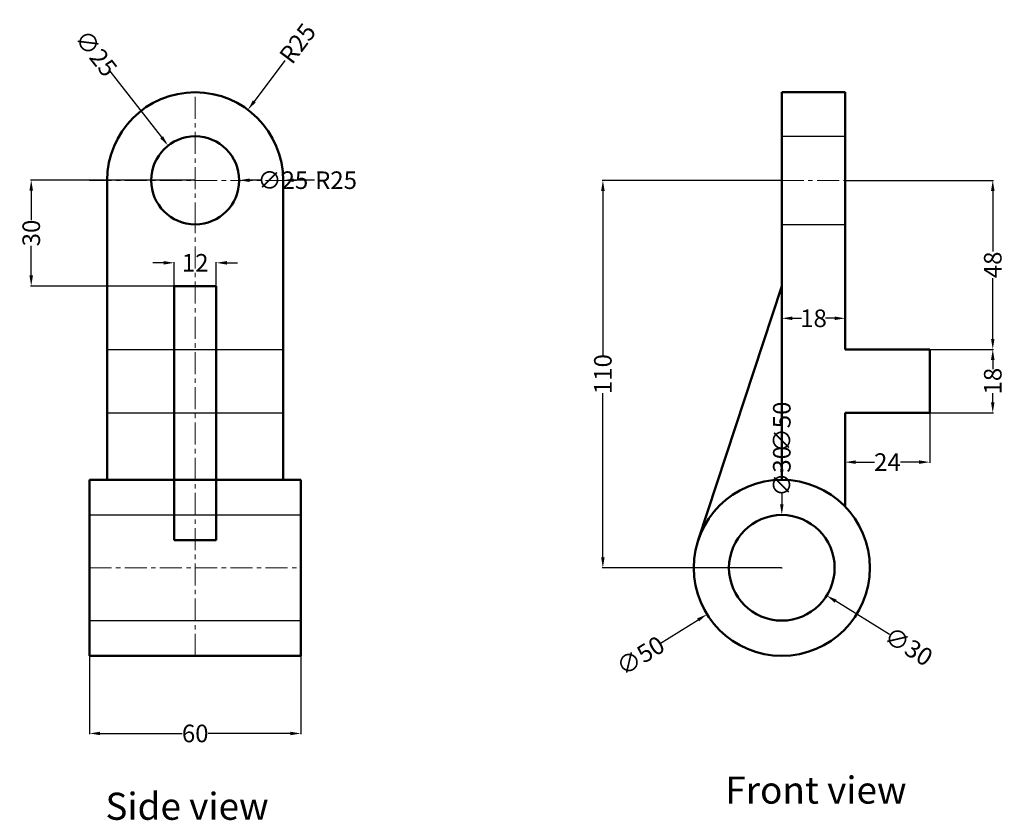
# Model space of a CAD drawing. Units: inches. Extents: x 36 to 316, y 40 to 267.
import ezdxf

# ---------------------------------------------------------------- set-up
doc = ezdxf.new("R2010")
doc.units = ezdxf.units.IN
doc.header["$MEASUREMENT"] = 0
doc.linetypes.add('CENTER', pattern=[2, 1.25, -0.25, 0.25, -0.25])
doc.linetypes.add('HIDDEN', pattern=[9.525, 6.35, -3.175])
for name, color, linetype, lineweight in [('M-CNTR', 4, 'CENTER', 18), ('M-DIMS', 2, 'Continuous', 25), ('M-HIDN', 3, 'HIDDEN', 25), ('M-OUTL', 7, 'Continuous', 50), ('M-TEXT', 7, 'Continuous', 25)]:
    doc.layers.add(name, color=color, linetype=linetype, lineweight=lineweight)
doc.styles.get("Standard").update_dxf_attribs({"font": 'arial.ttf'})
doc.dimstyles.get("Standard").update_dxf_attribs({"dimtxt": 5, "dimasz": 3, "dimexe": 0.18, "dimexo": 0.0625, "dimgap": 0.09, "dimtad": 0, "dimdec": 0, "dimzin": 0, "dimdsep": 46, "dimtxsty": 'Standard', "dimcen": 0.09, "dimadec": 0, "dimazin": 0, "dimtfac": 1, "dimtdec": 0, "dimtofl": 0, "dimtmove": 0, "dimatfit": 3, "dimfxl": 1, "dimtolj": 1, "dimtzin": 0, "dimarcsym": 0})

# ---------------------------------------------------------------- blocks, each defined once
blk = doc.blocks.new('*D1')
at = {"layer": 'Defpoints', "color": 0, "transparency": 16777216}
for p in [(252.72, 221.19), (201.9, 111.19), (252.72, 111.19)]:
    blk.add_point(p, dxfattribs=at)
at = {"layer": 'M-DIMS', "color": 0, "lineweight": -2, "transparency": 16777216}
for p, q in [((252.66, 221.19), (201.72, 221.19)), ((201.9, 218.19), (201.9, 171.56)), ((201.9, 114.19), (201.9, 160.82)), ((252.66, 111.19), (201.72, 111.19))]:
    blk.add_line(p, q, dxfattribs=at)
at = {"layer": 'M-DIMS', "color": 0, "transparency": 16777216}
for points in [[(201.4, 218.19), (202.4, 218.19), (201.9, 221.19)], [(201.4, 114.19), (202.4, 114.19), (201.9, 111.19)]]:
    blk.add_solid(points, dxfattribs=at)
at = {"layer": 'M-DIMS', "color": 0, "transparency": 16777216, "insert": (201.9, 166.19), "char_height": 5, "attachment_point": 5, "rotation": 90}
blk.add_mtext('\\A1;110', dxfattribs=at)
blk = doc.blocks.new('*D2')
at = {"layer": 'Defpoints', "color": 0, "transparency": 16777216}
for p in [(273.96, 124.39), (231.49, 98)]:
    blk.add_point(p, dxfattribs=at)
at = {"layer": 'M-DIMS', "color": 0, "lineweight": -2, "transparency": 16777216}
for p, q in [((252.63, 111.19), (252.81, 111.19)), ((252.72, 111.1), (252.72, 111.28)), ((217.99, 89.61), (228.94, 96.41))]:
    blk.add_line(p, q, dxfattribs=at)
at = {"layer": 'M-DIMS', "color": 0, "transparency": 16777216}
blk.add_solid([(228.68, 96.84), (229.2, 95.99), (231.49, 98)], dxfattribs=at)
at = {"layer": 'M-DIMS', "color": 0, "transparency": 16777216, "insert": (212.57, 86.24), "char_height": 5, "attachment_point": 5, "rotation": 31.8568}
blk.add_mtext('\\A1;∅50', dxfattribs=at)
blk = doc.blocks.new('*D3')
at = {"layer": 'Defpoints', "color": 0, "transparency": 16777216}
for p in [(239.97, 119.09), (265.48, 103.3)]:
    blk.add_point(p, dxfattribs=at)
at = {"layer": 'M-DIMS', "color": 0, "lineweight": -2, "transparency": 16777216}
for p, q in [((252.63, 111.19), (252.81, 111.19)), ((252.72, 111.1), (252.72, 111.28)), ((283.31, 92.25), (268.03, 101.72))]:
    blk.add_line(p, q, dxfattribs=at)
at = {"layer": 'M-DIMS', "color": 0, "transparency": 16777216}
blk.add_solid([(268.29, 102.14), (267.76, 101.29), (265.48, 103.3)], dxfattribs=at)
at = {"layer": 'M-DIMS', "color": 0, "transparency": 16777216, "insert": (288.74, 88.89), "char_height": 5, "attachment_point": 5, "rotation": 328.2295}
blk.add_mtext('\\A1;∅30', dxfattribs=at)
blk = doc.blocks.new('*D4')
at = {"layer": 'Defpoints', "color": 0, "transparency": 16777216}
for p in [(294.72, 173.19), (312.64, 173.19), (294.72, 155.19)]:
    blk.add_point(p, dxfattribs=at)
at = {"layer": 'M-DIMS', "color": 0, "lineweight": -2, "transparency": 16777216}
for p, q in [((294.79, 173.19), (312.82, 173.19)), ((312.64, 170.19), (312.64, 167.63)), ((312.64, 158.19), (312.64, 160.75)), ((294.79, 155.19), (312.82, 155.19))]:
    blk.add_line(p, q, dxfattribs=at)
at = {"layer": 'M-DIMS', "color": 0, "transparency": 16777216}
for points in [[(312.14, 170.19), (313.14, 170.19), (312.64, 173.19)], [(312.14, 158.19), (313.14, 158.19), (312.64, 155.19)]]:
    blk.add_solid(points, dxfattribs=at)
at = {"layer": 'M-DIMS', "color": 0, "transparency": 16777216, "insert": (312.64, 164.19), "char_height": 5, "attachment_point": 5, "rotation": 90}
blk.add_mtext('\\A1;18', dxfattribs=at)
blk = doc.blocks.new('*D5')
at = {"layer": 'Defpoints', "color": 0, "transparency": 16777216}
for p in [(270.72, 155.19), (294.72, 155.19), (294.72, 141.2)]:
    blk.add_point(p, dxfattribs=at)
at = {"layer": 'M-DIMS', "color": 0, "lineweight": -2, "transparency": 16777216}
for p, q in [((270.72, 155.13), (270.72, 141.02)), ((294.72, 155.13), (294.72, 141.02)), ((273.72, 141.2), (279.02, 141.2)), ((291.72, 141.2), (286.43, 141.2))]:
    blk.add_line(p, q, dxfattribs=at)
at = {"layer": 'M-DIMS', "color": 0, "transparency": 16777216}
for points in [[(273.72, 141.7), (273.72, 140.7), (270.72, 141.2)], [(291.72, 141.7), (291.72, 140.7), (294.72, 141.2)]]:
    blk.add_solid(points, dxfattribs=at)
at = {"layer": 'M-DIMS', "color": 0, "transparency": 16777216, "insert": (282.72, 141.2), "char_height": 5, "attachment_point": 5}
blk.add_mtext('\\A1;24', dxfattribs=at)
blk = doc.blocks.new('*D6')
at = {"layer": 'Defpoints', "color": 0, "transparency": 16777216}
for p in [(270.72, 221.19), (270.72, 173.19), (312.64, 173.19)]:
    blk.add_point(p, dxfattribs=at)
at = {"layer": 'M-DIMS', "color": 0, "lineweight": -2, "transparency": 16777216}
for p, q in [((270.79, 221.19), (312.82, 221.19)), ((312.64, 218.19), (312.64, 200.97)), ((312.64, 176.19), (312.64, 193.42)), ((270.79, 173.19), (312.82, 173.19))]:
    blk.add_line(p, q, dxfattribs=at)
at = {"layer": 'M-DIMS', "color": 0, "transparency": 16777216}
for points in [[(312.14, 218.19), (313.14, 218.19), (312.64, 221.19)], [(312.14, 176.19), (313.14, 176.19), (312.64, 173.19)]]:
    blk.add_solid(points, dxfattribs=at)
at = {"layer": 'M-DIMS', "color": 0, "transparency": 16777216, "insert": (312.64, 197.19), "char_height": 5, "attachment_point": 5, "rotation": 90}
blk.add_mtext('\\A1;48', dxfattribs=at)
blk = doc.blocks.new('*D7')
at = {"layer": 'Defpoints', "color": 0, "transparency": 16777216}
for p in [(252.72, 182.03), (252.72, 173.19), (270.72, 173.19)]:
    blk.add_point(p, dxfattribs=at)
at = {"layer": 'M-DIMS', "color": 0, "lineweight": -2, "transparency": 16777216}
for p, q in [((252.72, 173.26), (252.72, 182.21)), ((255.72, 182.03), (258.28, 182.03)), ((267.72, 182.03), (265.16, 182.03)), ((270.72, 173.26), (270.72, 182.21))]:
    blk.add_line(p, q, dxfattribs=at)
at = {"layer": 'M-DIMS', "color": 0, "transparency": 16777216}
for points in [[(255.72, 182.53), (255.72, 181.53), (252.72, 182.03)], [(267.72, 182.53), (267.72, 181.53), (270.72, 182.03)]]:
    blk.add_solid(points, dxfattribs=at)
at = {"layer": 'M-DIMS', "color": 0, "transparency": 16777216, "insert": (261.72, 182.03), "char_height": 5, "attachment_point": 5}
blk.add_mtext('\\A1;18', dxfattribs=at)
blk = doc.blocks.new('*D8')
at = {"layer": 'Defpoints', "color": 0, "transparency": 16777216}
for p in [(101.09, 241.21), (86.11, 221.19)]:
    blk.add_point(p, dxfattribs=at)
at = {"layer": 'M-DIMS', "color": 0, "lineweight": -2, "transparency": 16777216}
for p, q in [((111.56, 255.2), (102.89, 243.61)), ((86.02, 221.19), (86.2, 221.19)), ((86.11, 221.1), (86.11, 221.28))]:
    blk.add_line(p, q, dxfattribs=at)
at = {"layer": 'M-DIMS', "color": 0, "transparency": 16777216}
blk.add_solid([(102.49, 243.91), (103.29, 243.31), (101.09, 241.21)], dxfattribs=at)
at = {"layer": 'M-DIMS', "color": 0, "transparency": 16777216, "insert": (115.2, 260.07), "char_height": 5, "attachment_point": 5, "rotation": 53.1928}
blk.add_mtext('\\A1;R25', dxfattribs=at)
blk = doc.blocks.new('*D9')
at = {"layer": 'Defpoints', "color": 0, "transparency": 16777216}
for p in [(78.42, 231.05), (93.81, 211.34)]:
    blk.add_point(p, dxfattribs=at)
at = {"layer": 'M-DIMS', "color": 0, "lineweight": -2, "transparency": 16777216}
for p, q in [((61.89, 252.22), (76.58, 233.41)), ((86.02, 221.19), (86.2, 221.19)), ((86.11, 221.1), (86.11, 221.28))]:
    blk.add_line(p, q, dxfattribs=at)
at = {"layer": 'M-DIMS', "color": 0, "transparency": 16777216}
blk.add_solid([(76.97, 233.72), (76.18, 233.1), (78.42, 231.05)], dxfattribs=at)
at = {"layer": 'M-DIMS', "color": 0, "transparency": 16777216, "insert": (57.95, 257.27), "char_height": 5, "attachment_point": 5, "rotation": 307.9788}
blk.add_mtext('\\A1;∅25', dxfattribs=at)
blk = doc.blocks.new('*D10')
at = {"layer": 'Defpoints', "color": 0, "transparency": 16777216}
for p in [(86.11, 221.28), (39.54, 191.19), (86.11, 191.19)]:
    blk.add_point(p, dxfattribs=at)
at = {"layer": 'M-DIMS', "color": 0, "lineweight": -2, "transparency": 16777216}
for p, q in [((86.05, 221.28), (39.36, 221.28)), ((39.54, 218.28), (39.54, 209.9)), ((39.54, 194.19), (39.54, 202.58)), ((86.05, 191.19), (39.36, 191.19))]:
    blk.add_line(p, q, dxfattribs=at)
at = {"layer": 'M-DIMS', "color": 0, "transparency": 16777216}
for points in [[(39.04, 218.28), (40.04, 218.28), (39.54, 221.28)], [(39.04, 194.19), (40.04, 194.19), (39.54, 191.19)]]:
    blk.add_solid(points, dxfattribs=at)
at = {"layer": 'M-DIMS', "color": 0, "transparency": 16777216, "insert": (39.54, 206.24), "char_height": 5, "attachment_point": 5, "rotation": 90}
blk.add_mtext('\\A1;30', dxfattribs=at)
blk = doc.blocks.new('*D11')
at = {"layer": 'Defpoints', "color": 0, "transparency": 16777216}
for p in [(92.11, 197.78), (80.11, 191.19), (92.11, 191.19)]:
    blk.add_point(p, dxfattribs=at)
at = {"layer": 'M-DIMS', "color": 0, "lineweight": -2, "transparency": 16777216}
for p, q in [((77.11, 197.78), (74.11, 197.78)), ((80.11, 191.26), (80.11, 197.96)), ((92.11, 191.26), (92.11, 197.96)), ((95.11, 197.78), (98.11, 197.78))]:
    blk.add_line(p, q, dxfattribs=at)
at = {"layer": 'M-DIMS', "color": 0, "transparency": 16777216}
for points in [[(77.11, 198.28), (77.11, 197.28), (80.11, 197.78)], [(95.11, 198.28), (95.11, 197.28), (92.11, 197.78)]]:
    blk.add_solid(points, dxfattribs=at)
at = {"layer": 'M-DIMS', "color": 0, "transparency": 16777216, "insert": (86.11, 197.78), "char_height": 5, "attachment_point": 5}
blk.add_mtext('\\A1;12', dxfattribs=at)
blk = doc.blocks.new('*D12')
at = {"layer": 'Defpoints', "color": 0, "transparency": 16777216}
for p in [(56.11, 86.19), (116.11, 86.19), (116.11, 64.17)]:
    blk.add_point(p, dxfattribs=at)
at = {"layer": 'M-DIMS', "color": 0, "lineweight": -2, "transparency": 16777216}
for p, q in [((56.11, 86.13), (56.11, 63.99)), ((116.11, 86.13), (116.11, 63.99)), ((59.11, 64.17), (82.44, 64.17)), ((113.11, 64.17), (89.79, 64.17))]:
    blk.add_line(p, q, dxfattribs=at)
at = {"layer": 'M-DIMS', "color": 0, "transparency": 16777216}
for points in [[(59.11, 64.67), (59.11, 63.67), (56.11, 64.17)], [(113.11, 64.67), (113.11, 63.67), (116.11, 64.17)]]:
    blk.add_solid(points, dxfattribs=at)
at = {"layer": 'M-DIMS', "color": 0, "transparency": 16777216, "insert": (86.11, 64.17), "char_height": 5, "attachment_point": 5}
blk.add_mtext('\\A1;60', dxfattribs=at)
blk = doc.blocks.new('*D13')
at = {"layer": 'Defpoints', "color": 0, "transparency": 16777216}
for p in [(86.11, 221.19), (111.11, 221.22)]:
    blk.add_point(p, dxfattribs=at)
at = {"layer": 'M-DIMS', "color": 0, "lineweight": -2, "transparency": 16777216}
for p, q in [((86.02, 221.19), (86.2, 221.19)), ((86.11, 221.1), (86.11, 221.28)), ((120.03, 221.22), (114.11, 221.22))]:
    blk.add_line(p, q, dxfattribs=at)
at = {"layer": 'M-DIMS', "color": 0, "transparency": 16777216}
blk.add_solid([(114.11, 221.72), (114.12, 220.72), (111.11, 221.22)], dxfattribs=at)
at = {"layer": 'M-DIMS', "color": 0, "transparency": 16777216, "insert": (126.11, 221.23), "char_height": 5, "attachment_point": 5, "rotation": 0.0502}
blk.add_mtext('\\A1;R25', dxfattribs=at)
blk = doc.blocks.new('*D14')
at = {"layer": 'Defpoints', "color": 0, "transparency": 16777216}
for p in [(73.61, 221.17), (98.61, 221.21)]:
    blk.add_point(p, dxfattribs=at)
at = {"layer": 'M-DIMS', "color": 0, "lineweight": -2, "transparency": 16777216}
for p, q in [((86.02, 221.19), (86.2, 221.19)), ((86.11, 221.1), (86.11, 221.28)), ((104.61, 221.23), (101.61, 221.22))]:
    blk.add_line(p, q, dxfattribs=at)
at = {"layer": 'M-DIMS', "color": 0, "transparency": 16777216}
blk.add_solid([(101.61, 221.72), (101.62, 220.72), (98.61, 221.21)], dxfattribs=at)
at = {"layer": 'M-DIMS', "color": 0, "transparency": 16777216, "insert": (111.02, 221.24), "char_height": 5, "attachment_point": 5, "rotation": 0.1004}
blk.add_mtext('\\A1;∅25', dxfattribs=at)
blk = doc.blocks.new('*D15')
at = {"layer": 'Defpoints', "color": 0, "transparency": 16777216}
for p in [(252.72, 136.19), (252.72, 86.19)]:
    blk.add_point(p, dxfattribs=at)
at = {"layer": 'M-DIMS', "color": 0, "lineweight": -2, "transparency": 16777216}
for p, q in [((252.72, 144.81), (252.72, 139.19)), ((252.63, 111.19), (252.81, 111.19)), ((252.72, 111.1), (252.72, 111.28))]:
    blk.add_line(p, q, dxfattribs=at)
at = {"layer": 'M-DIMS', "color": 0, "transparency": 16777216}
blk.add_solid([(252.22, 139.19), (253.22, 139.19), (252.72, 136.19)], dxfattribs=at)
at = {"layer": 'M-DIMS', "color": 0, "transparency": 16777216, "insert": (252.72, 151.19), "char_height": 5, "attachment_point": 5, "rotation": 89.9996}
blk.add_mtext('\\A1;∅50', dxfattribs=at)
blk = doc.blocks.new('*D16')
at = {"layer": 'Defpoints', "color": 0, "transparency": 16777216}
for p in [(252.72, 126.19), (252.72, 96.19)]:
    blk.add_point(p, dxfattribs=at)
at = {"layer": 'M-DIMS', "color": 0, "lineweight": -2, "transparency": 16777216}
for p, q in [((252.72, 132.19), (252.72, 129.19)), ((252.63, 111.19), (252.81, 111.19)), ((252.72, 111.1), (252.72, 111.28))]:
    blk.add_line(p, q, dxfattribs=at)
at = {"layer": 'M-DIMS', "color": 0, "transparency": 16777216}
blk.add_solid([(252.22, 129.19), (253.22, 129.19), (252.72, 126.19)], dxfattribs=at)
at = {"layer": 'M-DIMS', "color": 0, "transparency": 16777216, "insert": (252.72, 138.58), "char_height": 5, "attachment_point": 5, "rotation": 89.9993}
blk.add_mtext('\\A1;∅30', dxfattribs=at)

msp = doc.modelspace()

# ---------------------------------------------------------------- linework, layer by layer
at = {"layer": 'M-CNTR', "ltscale": 5}
for p, q in [((86.11, 208.69), (86.11, 246.19)), ((56.11, 221.19), (116.11, 221.19)), ((252.72, 221.19), (270.72, 221.19)), ((86.11, 86.19), (86.11, 208.69)), ((56.11, 111.19), (116.11, 111.19))]:
    msp.add_line(p, q, dxfattribs=at)
at = {"layer": 'M-HIDN', "ltscale": 10}
for p, q in [((252.72, 233.69), (270.72, 233.69)), ((252.72, 208.69), (270.72, 208.69)), ((61.11, 173.19), (111.11, 173.19)), ((61.11, 155.19), (111.11, 155.19)), ((56.11, 126.19), (116.11, 126.19)), ((56.11, 96.19), (116.11, 96.19))]:
    msp.add_line(p, q, dxfattribs=at)
at = {"layer": 'M-OUTL'}
for p, q in [((252.72, 136.19), (252.72, 246.19)), ((252.72, 246.19), (270.72, 246.19)), ((270.72, 173.19), (270.72, 246.19)), ((61.11, 136.19), (61.11, 221.19)), ((111.11, 136.19), (111.11, 221.19)), ((92.11, 191.19), (80.11, 191.19)), ((80.11, 119.01), (80.11, 191.19)), ((92.11, 119.01), (92.11, 191.19)), ((252.72, 191.19), (228.97, 119.01)), ((270.72, 173.19), (294.72, 173.19)), ((294.72, 155.19), (294.72, 173.19)), ((270.72, 128.54), (270.72, 155.19)), ((270.72, 155.19), (294.72, 155.19)), ((56.11, 86.19), (56.11, 136.19)), ((56.11, 136.19), (116.11, 136.19)), ((116.11, 86.19), (116.11, 136.19)), ((92.11, 119.01), (80.11, 119.01)), ((56.11, 86.19), (116.11, 86.19))]:
    msp.add_line(p, q, dxfattribs=at)
for centre, radius in [((86.11, 221.19), 12.5), ((252.72, 111.19), 25), ((252.72, 111.19), 15)]:
    msp.add_circle(centre, radius, dxfattribs=at)
for start, end in [(90, 180), (0, 90)]:
    msp.add_arc((86.11, 221.19), 25, start, end, dxfattribs=at)

# ---------------------------------------------------------------- texts
at = {"layer": 'M-TEXT', "char_height": 7.685, "attachment_point": 1}
for s, insert in [('Front view', (236.69, 51.93)), ('Side view', (60.61, 47.34))]:
    msp.add_mtext_dynamic_manual_height_columns(s, width=75.585, gutter_width=0.769, heights=[0], dxfattribs=dict(at, insert=insert))

# ---------------------------------------------------------------- dimensions: what is measured, and where the dimension line sits
at = {"layer": 'M-DIMS'}
for mpoint, override, picture, middle in [((101.09, 241.21), {"dimclrd": 0, "dimclre": 0, "dimclrt": 0}, '*D8', (115.2, 260.07)), ((111.11, 221.21), {"dimdec": 0, "dimlfac": 1, "dimrnd": 0, "dimzin": 0, "dimdsep": 46, "dimlunit": 2}, '*D13', (126.11, 221.23))]:
    dim = msp.add_radius_dim(center=(86.11, 221.19), mpoint=mpoint, dimstyle='Standard', override=override, dxfattribs=at)
    dim.commit()
    dim.dimension.update_dxf_attribs({"geometry": picture, "text_midpoint": middle, "dimtype": 164})
for p1, p2, override, picture, middle in [((93.81, 211.34), (78.42, 231.05), {"dimclrd": 0, "dimclre": 0, "dimclrt": 0}, '*D9', (57.95, 257.27)), ((252.72, 86.19), (252.72, 136.19), {"dimdec": 0, "dimlfac": 1, "dimrnd": 0, "dimzin": 0, "dimdsep": 46, "dimlunit": 2}, '*D15', (252.72, 151.19)), ((273.96, 124.39), (231.49, 98), {"dimclrd": 0, "dimclre": 0, "dimclrt": 0}, '*D2', (212.57, 86.24)), ((239.97, 119.09), (265.48, 103.3), {"dimclrd": 0, "dimclre": 0, "dimclrt": 0}, '*D3', (288.74, 88.89))]:
    dim = msp.add_diameter_dim_2p(p1=p1, p2=p2, dimstyle='Standard', override=override, dxfattribs=at)
    dim.commit()
    dim.dimension.update_dxf_attribs({"geometry": picture, "text_midpoint": middle, "dimtype": 163})
for p1, p2, picture, middle in [((73.61, 221.17), (98.61, 221.21), '*D14', (111.02, 221.24)), ((252.72, 96.19), (252.72, 126.19), '*D16', (252.72, 138.58))]:
    dim = msp.add_diameter_dim_2p(p1=p1, p2=p2, dimstyle='Standard', override={"dimdec": 0, "dimlfac": 1, "dimrnd": 0, "dimzin": 0, "dimdsep": 46, "dimlunit": 2}, dxfattribs=at)
    dim.commit()
    dim.dimension.update_dxf_attribs({"geometry": picture, "text_midpoint": middle})
for base, p1, p2, picture, middle in [((39.54, 191.19), (86.11, 221.28), (86.11, 191.19), '*D10', (39.54, 206.24)), ((201.9, 111.19), (252.72, 221.19), (252.72, 111.19), '*D1', (201.9, 166.19)), ((312.64, 173.19), (270.72, 221.19), (270.72, 173.19), '*D6', (312.64, 197.19)), ((312.64, 173.19), (294.72, 155.19), (294.72, 173.19), '*D4', (312.64, 164.19))]:
    dim = msp.add_linear_dim(base=base, p1=p1, p2=p2, angle=90, dimstyle='Standard', override={"dimclrd": 0, "dimclre": 0, "dimclrt": 0}, dxfattribs=at)
    dim.commit()
    dim.dimension.update_dxf_attribs({"geometry": picture, "text_midpoint": middle})
for base, p1, p2, picture, middle in [((92.11, 197.78), (80.11, 191.19), (92.11, 191.19), '*D11', (86.11, 197.78)), ((294.72, 141.2), (270.72, 155.19), (294.72, 155.19), '*D5', (282.72, 141.2)), ((116.11, 64.17), (56.11, 86.19), (116.11, 86.19), '*D12', (86.11, 64.17))]:
    dim = msp.add_linear_dim(base=base, p1=p1, p2=p2, dimstyle='Standard', override={"dimclrd": 0, "dimclre": 0, "dimclrt": 0}, dxfattribs=at)
    dim.commit()
    dim.dimension.update_dxf_attribs({"geometry": picture, "text_midpoint": middle})
dim = msp.add_linear_dim(base=(252.72, 182.03), p1=(270.72, 173.19), p2=(252.72, 173.19), dimstyle='Standard', override={"dimclrd": 0, "dimclre": 0, "dimclrt": 0}, dxfattribs=at)
dim.commit()
dim.dimension.update_dxf_attribs({"geometry": '*D7', "text_midpoint": (261.72, 182.03), "dimtype": 160})

doc.saveas('drawing.dxf')
